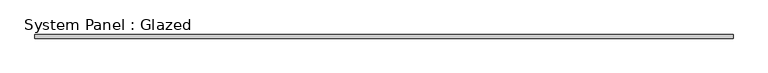
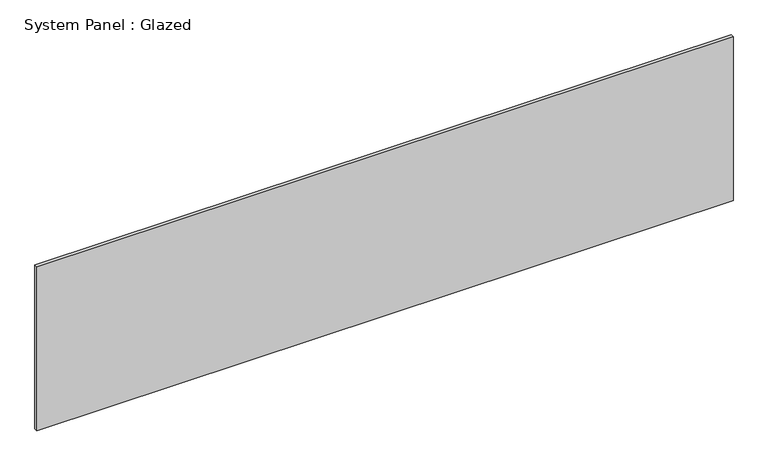
"""IFC4 building model written with IfcOpenShell, lengths in millimetres: plate geometry, System Panel : Glazed."""

from ifc_helpers import new_model, si_unit, origin, origin_with_axes, place, context, project, spatial, polyline, outline, extrude, source, transform, mapped, element, save


def system_panel_glazed_3a47dc32(model_context):
    return source(origin(), model_context, "Body", "SweptSolid", [
        extrude(outline(polyline([(2451.8626044, 19.05), (-2451.8626044, 19.05), (-2451.8626044, 44.45), (2451.8626044, 44.45), (2451.8626044, 19.05)])), origin_with_axes(), (0.0, 0.0, 1.0), 1219.2),
    ])


if __name__ == "__main__":
    model = new_model("IFC4")
    model_context = context("Model", 3, world=origin())
    ifc_project = project(units=[si_unit("LENGTHUNIT", "METRE", prefix="MILLI")], contexts=[model_context])
    site = spatial("IfcSite", under=ifc_project)
    building = spatial("IfcBuilding", under=site)
    placement = place(None, origin())
    system_panel_glazed_shape = system_panel_glazed_3a47dc32(model_context)
    element("IfcPlate", 1, ObjectType="System Panel : Glazed", at=placement, inside=building, context=model_context, shape_type="MappedRepresentation", body=[
        mapped(system_panel_glazed_shape, transform((0.0, 0.0, 0.0), x_axis=(1.0, 0.0, 0.0), y_axis=(0.0, 1.0, 0.0), z_axis=(0.0, 0.0, 1.0))),
    ])
    save(model, "model.ifc")

# Revit data of these elements
# Type "System Panel : Glazed"
#   Construction Type Id = "GSP4R"
#   Analytic Construction = "1/8 in Pilkington single glazing"
#   Visual Light Transmittance = 0.9
#   Solar Heat Gain Coefficient = 0.86
#   Heat Transfer Coefficient (U) = 1.18115 BTU/(h·ft²·°F)
# Element 1 (IfcPlate, "System Panel : Glazed")
#   Materials on its faces: "Glass"
# Materials
#   "Glass": class "Glass", colour RGB 0 128 192, transparency 0.75, Description = "Soda Lime Glass", Cost = 0
